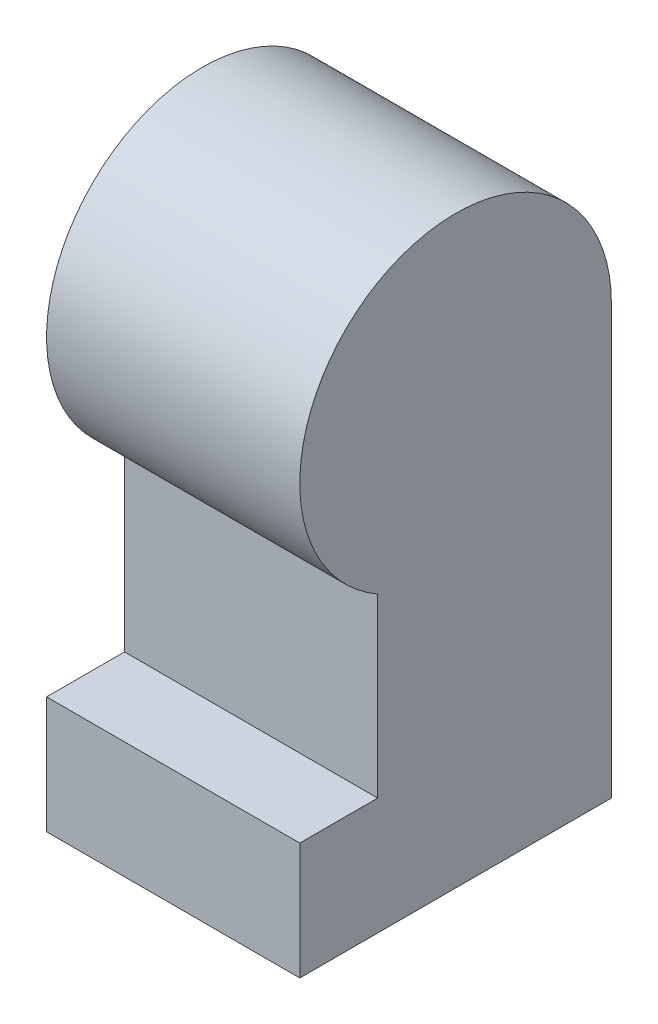
SolidWorks part; units mm, degrees
material "Plain Carbon Steel"
ref_plane "Front Plane" through (0, 0, 0) normal (0, 0, 1) x (1, 0, 0)
ref_plane "Top Plane" through (0, 0, 0) normal (0, 1, 0) x (1, 0, 0)
ref_plane "Right Plane" through (0, 0, 0) normal (1, 0, 0) x (0, 0, -1)
sketch "Leg Profile Sketch" plane through (0, 0, 0) normal (1, 0, 0) x (0, 0, -1)
  line L0 (4, 0) -> (4, -11)
  line L1 (4, -11) -> (-4, -11)
  line L2 (-4, -11) -> (-4, -8)
  line L3 (-4, -8) -> (-2, -8)
  line L4 (-2, -8) -> (-2, -3.4641)
  arc A0 (4, 0) -> (-2, -3.4641) centre (0, 0) ccw
  dimension "D1" = 8
  dimension "D2" = 11
  dimension "D3" = 8
  dimension "D4" = 3
  dimension "D5" = 2
extrude "Leg Body" add sketch "Leg Profile Sketch" along normal mid plane 6.5
shell "Leg Shell 1mm" thickness 1
sketch "Hip Pin Hole Sketch" plane through (-3.25, 0, 0) normal (-1, 0, 0) x (0, 0, 1)
  circle A0 centre (0, 0) radius 1.5
  dimension "D1" = 3
extrude "Hip Pin Hole Ø3" cut sketch "Hip Pin Hole Sketch" against normal up to next
